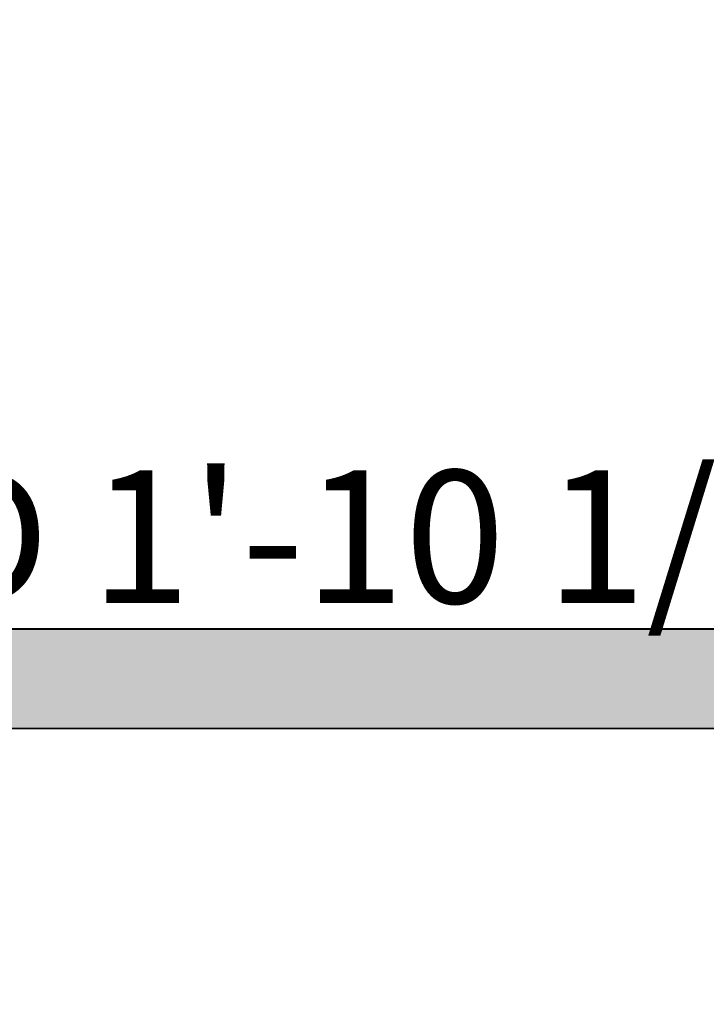
# Model space of a CAD drawing. Units: inches. Extents: x 2083 to 3317, y 1141 to 2115.
# Tile 118 of 256: x 2944 to 3006, y 1238 to 1327. Entities that reach past the tile are written whole.
import ezdxf

# ---------------------------------------------------------------- set-up
doc = ezdxf.new("R2010")
doc.units = ezdxf.units.IN
doc.layers.add('A-ANNO-DIMS', color=2, linetype='Continuous', lineweight=18)
doc.layers.add('A-WALL', color=7, linetype='Continuous', lineweight=35)
doc.layers.add('A-WALL-PATT', color=251, linetype='Continuous', lineweight=13, true_color=0x636466)
doc.styles.get("Standard").update_dxf_attribs({"font": 'arial.ttf'})
doc.dimstyles.new('ISO-25', dxfattribs={"dimtxt": 12, "dimasz": 12, "dimexe": 1.25, "dimexo": 0.625, "dimtad": 1, "dimlunit": 3, "dimtxsty": 'Standard', "dimcen": 2.5, "dimadec": 0, "dimazin": 0, "dimtfac": 1, "dimtmove": 0, "dimatfit": 3, "dimfxl": 1, "dimarcsym": 0})

# ---------------------------------------------------------------- blocks, each defined once
blk = doc.blocks.new('*D10')
at = {"layer": 'A-ANNO-DIMS', "color": 0, "lineweight": -2, "transparency": 16777216}
for p, q in [((2862.96, 1262.636), (2862.96, 1201.384)), ((3126.96, 1262.636), (3126.96, 1201.384)), ((2874.96, 1202.634), (3114.96, 1202.634))]:
    blk.add_line(p, q, dxfattribs=at)
at = {"layer": 'A-ANNO-DIMS', "color": 0, "transparency": 16777216}
for points in [[(2874.96, 1204.634), (2874.96, 1200.634), (2862.96, 1202.634)], [(3114.96, 1204.634), (3114.96, 1200.634), (3126.96, 1202.634)]]:
    blk.add_solid(points, dxfattribs=at)
at = {"layer": 'Defpoints', "color": 0, "transparency": 16777216}
for p in [(2862.96, 1263.261), (3126.96, 1263.261), (3126.96, 1202.634)]:
    blk.add_point(p, dxfattribs=at)
at = {"layer": 'A-ANNO-DIMS', "color": 0, "transparency": 16777216, "insert": (2994.96, 1209.284), "char_height": 12, "attachment_point": 5}
blk.add_mtext("22'", dxfattribs=at)
blk = doc.blocks.new('*D26')
at = {"layer": 'A-ANNO-DIMS', "color": 0, "lineweight": -2, "transparency": 16777216}
for p, q in [((3088.986, 1274.915), (3088.986, 1270.952)), ((3111.24, 1274.915), (3111.24, 1270.952)), ((3076.986, 1272.202), (2840.262, 1272.202)), ((3111.24, 1272.202), (3088.986, 1272.202)), ((3123.24, 1272.202), (3135.24, 1272.202))]:
    blk.add_line(p, q, dxfattribs=at)
at = {"layer": 'A-ANNO-DIMS', "color": 0, "transparency": 16777216}
for points in [[(3076.986, 1274.202), (3076.986, 1270.202), (3088.986, 1272.202)], [(3123.24, 1274.202), (3123.24, 1270.202), (3111.24, 1272.202)]]:
    blk.add_solid(points, dxfattribs=at)
at = {"layer": 'Defpoints', "color": 0, "transparency": 16777216}
for p in [(3088.986, 1275.54), (3111.24, 1275.54), (3088.986, 1272.202)]:
    blk.add_point(p, dxfattribs=at)
at = {"layer": 'A-ANNO-DIMS', "color": 0, "transparency": 16777216, "insert": (2952.624, 1279.032), "char_height": 12, "attachment_point": 5}
blk.add_mtext('NIGHTSTAND 1\'-10 1/2" TYP.', dxfattribs=at)
blk = doc.blocks.new('*D34')
at = {"layer": 'A-ANNO-DIMS', "color": 0, "lineweight": -2, "transparency": 16777216}
for p, q in [((2226.96, 1262.636), (2226.96, 1209.661)), ((3126.96, 1262.636), (3126.96, 1209.661)), ((2238.96, 1210.911), (3114.96, 1210.911))]:
    blk.add_line(p, q, dxfattribs=at)
at = {"layer": 'A-ANNO-DIMS', "color": 0, "transparency": 16777216}
for points in [[(2238.96, 1212.911), (2238.96, 1208.911), (2226.96, 1210.911)], [(3114.96, 1212.911), (3114.96, 1208.911), (3126.96, 1210.911)]]:
    blk.add_solid(points, dxfattribs=at)
at = {"layer": 'Defpoints', "color": 0, "transparency": 16777216}
for p in [(2226.96, 1263.261), (3126.96, 1263.261), (3126.96, 1210.911)]:
    blk.add_point(p, dxfattribs=at)
at = {"layer": 'A-ANNO-DIMS', "color": 0, "transparency": 16777216, "insert": (2676.96, 1217.663), "char_height": 12, "attachment_point": 5}
blk.add_mtext('75\'-0"', dxfattribs=at)

msp = doc.modelspace()

# ---------------------------------------------------------------- hatches: boundary and pattern name
at = {"layer": 'A-WALL-PATT'}
h = msp.add_hatch(color=256, dxfattribs=at)
h.dxf.hatch_style = 1
h.paths.add_polyline_path([(3126.96, 2020.761), (2748.96, 2020.761), (2604.96, 2020.761), (2226.96, 2020.761), (2226.96, 1702.761), (2466.96, 1702.761), (2466.96, 1582.761), (2418.96, 1582.761), (2418.96, 1477.761), (2226.96, 1477.761), (2226.96, 1263.261), (2544.96, 1263.261), (2544.96, 1411.761), (2604.96, 1411.761), (2685.96, 1411.761), (2685.96, 1420.761), (2604.96, 1420.761), (2604.96, 1573.761), (2604.96, 1702.761), (2604.96, 2011.761), (2748.96, 2011.761), (2748.96, 1702.761), (2862.96, 1702.761), (2862.96, 1621.761), (2871.96, 1621.761), (2871.96, 1702.761), (2883.96, 1702.761), (2883.96, 1706.939, -0.026459), (2883.96, 1711.761), (2757.96, 1711.761), (2757.96, 1807.761), (2787.96, 1807.761), (2787.96, 1812.261), (2757.96, 1812.261), (2757.96, 2011.761), (2877.96, 2011.761), (2877.96, 1812.261), (2847.96, 1812.261), (2847.96, 1807.761), (2889.836, 1807.761), (2889.836, 1812.261), (2882.46, 1812.261), (2882.46, 2011.761), (3117.96, 2011.761), (3117.96, 1812.261), (2937.836, 1812.261), (2937.836, 1807.761), (2995.71, 1807.761), (2995.71, 1796.118), (3000.21, 1796.118), (3000.21, 1807.761), (3117.96, 1807.761), (3117.96, 1711.761), (3000.21, 1711.761), (3000.21, 1760.118), (2998.573, 1760.118, -0.020711), (2995.71, 1760.118), (2995.71, 1711.761), (2931.96, 1711.761), (2931.96, 1702.761), (3126.96, 1702.761)])
h.paths.add_polyline_path([(2471.46, 2011.761), (2471.46, 1810.011), (2462.717, 1810.011), (2462.717, 1805.511), (2505.96, 1805.511), (2505.96, 1810.011), (2475.96, 1810.011), (2475.96, 2011.761), (2595.96, 2011.761), (2595.96, 1810.011), (2565.96, 1810.011), (2565.96, 1805.511), (2595.96, 1805.511), (2595.96, 1711.761), (2235.96, 1711.761), (2235.96, 1805.511), (2353.71, 1805.511), (2353.71, 1796.054), (2358.21, 1796.054), (2358.21, 1805.511), (2414.717, 1805.511), (2414.717, 1810.011), (2235.96, 1810.011), (2235.96, 2011.761)], flags=16)
h.paths.add_polyline_path([(2270.205, 1994.61), (2270.205, 1970.61), (2246.205, 1970.61), (2246.205, 1994.61)], flags=0)
edge = h.paths.add_edge_path(flags=0)
edge.add_ellipse((2332.027, 1899.798), major_axis=(-3.043, 3.043), ratio=0.168252, start_angle=-161.33217, end_angle=-156.30711, ccw=False)
edge.add_ellipse((2333.082, 1898.744), major_axis=(-1.055, 1.055), ratio=0.453532, start_angle=-123.37102, end_angle=-94.15911)
edge = h.paths.add_edge_path(flags=0)
edge.add_ellipse((2332.027, 1968.876), major_axis=(3.043, 3.043), ratio=0.168252, start_angle=18.66783, end_angle=23.69289)
edge.add_spline(control_points=[(2332.926, 1970.691), (2332.227, 1970.336), (2330.894, 1969.659), (2328.413, 1970.932), (2327.204, 1967.749), (2324.71, 1969.956), (2322.533, 1967.012), (2320.013, 1971.296), (2317.68, 1968.158), (2316.041, 1967.102), (2315.427, 1966.81)], knot_values=[0, 0, 0, 0, 2.267059, 4.324559, 6.685584, 8.878641, 11.121502, 14.300359, 17.755284, 19.732645, 19.732645, 19.732645, 19.732645], degree=3, periodic=0)
edge.add_ellipse((2332.027, 1968.876), major_axis=(3.043, 3.043), ratio=0.168252, start_angle=18.66783, end_angle=23.69289, ccw=False)
edge.add_ellipse((2333.082, 1969.931), major_axis=(1.055, 1.055), ratio=0.453532, start_angle=56.62898, end_angle=85.84089, ccw=False)
edge = h.paths.add_edge_path(flags=0)
edge.add_spline(control_points=[(2296.428, 1967.988), (2293.628, 1965.336), (2287.704, 1959.727), (2299.744, 1949.996), (2294.533, 1935.669), (2290.573, 1920.604), (2293.394, 1909.974), (2296.185, 1904.967)], knot_values=[0.099185, 0.099185, 0.099185, 0.099185, 0.345301, 0.619822, 0.982653, 1.386093, 1.810555, 1.810555, 1.810555, 1.810555], degree=3, periodic=0)
edge.add_spline(control_points=[(2296.185, 1904.967), (2297.384, 1902.619), (2298.001, 1901.949), (2298.553, 1901.468)], knot_values=[0.006246, 0.006246, 0.006246, 0.006246, 0.055476, 0.055476, 0.055476, 0.055476], degree=3, periodic=0)
edge.add_spline(control_points=[(2298.553, 1901.468), (2297.259, 1900.923), (2295.225, 1900.232), (2293.06, 1900.614), (2292.101, 1900.788), (2292.09, 1900.791)], knot_values=[0.312835, 0.312835, 0.312835, 0.312835, 0.40178, 0.474987, 0.475903, 0.475903, 0.475903, 0.475903], degree=3, periodic=0)
edge.add_arc((2292.794, 1904.664), 3.937, 215.4209, 259.69818, ccw=False)
edge.add_spline(control_points=[(2289.585, 1902.382), (2289.477, 1902.535), (2289.368, 1902.688), (2289.261, 1902.841)], knot_values=[0.102872, 0.102872, 0.102872, 0.102872, 0.116896, 0.116896, 0.116896, 0.116896], degree=3, periodic=0)
edge.add_spline(control_points=[(2289.261, 1902.841), (2288.687, 1902.55), (2287.64, 1902.02), (2285.881, 1901.874), (2283.853, 1901.504), (2281.72, 1899.711), (2278.467, 1899.493), (2276.157, 1901.883), (2272.259, 1899.804), (2267.778, 1901.843), (2262.244, 1900.184), (2257.415, 1901.782), (2254.318, 1900.726), (2253.178, 1900.337)], knot_values=[0, 0, 0, 0, 1.907977, 3.477176, 5.261074, 7.972851, 11.680248, 13.717921, 16.939592, 22.789562, 27.502503, 33.595215, 37.145618, 37.145618, 37.145618, 37.145618], degree=3, periodic=0)
edge.add_line((2253.178, 1900.337), (2250.244, 1902.841))
edge.add_line((2250.244, 1902.841), (2250.244, 1965.833))
edge.add_line((2250.244, 1965.833), (2253.178, 1968.337))
edge.add_spline(control_points=[(2253.178, 1968.337), (2254.318, 1967.948), (2257.415, 1966.892), (2262.244, 1968.49), (2267.778, 1966.831), (2271.527, 1968.537), (2273.876, 1967.828), (2274.207, 1967.728)], knot_values=[0, 0, 0, 0, 0.09018, 0.244935, 0.364644, 0.513233, 0.537855, 0.537855, 0.537855, 0.537855], degree=3, periodic=0)
edge.add_arc((2274.353, 1963.793), 3.937, 72.05113, 92.12795, ccw=False)
edge.add_arc((2281.297, 1985.23), 18.596, 252.05113, 288.56572)
edge.add_arc((2292.317, 1956.029), 12.646, 71.02679, 113.77822, ccw=False)
edge = h.paths.add_edge_path(flags=0)
edge.add_spline(control_points=[(2274.899, 1951.856), (2275.066, 1951.617), (2275.233, 1951.377), (2275.398, 1951.136)], knot_values=[1.409916, 1.409916, 1.409916, 1.409916, 1.43159, 1.43159, 1.43159, 1.43159], degree=3, periodic=0)
edge.add_spline(control_points=[(2275.398, 1951.136), (2275.792, 1950.562), (2276.179, 1949.984), (2276.546, 1949.397)], knot_values=[1.358238, 1.358238, 1.358238, 1.358238, 1.409916, 1.409916, 1.409916, 1.409916], degree=3, periodic=0)
edge.add_line((2276.546, 1949.397), (2277.437, 1947.862))
edge.add_spline(control_points=[(2277.437, 1947.862), (2276.304, 1945.673), (2274.64, 1942.427), (2274.632, 1938.094), (2272.799, 1930.852), (2274.356, 1943.897), (2275.948, 1947.923), (2276.546, 1949.397)], knot_values=[0.005632, 0.005632, 0.005632, 0.005632, 0.186014, 0.266002, 0.357087, 0.59639, 0.739732, 0.739732, 0.739732, 0.739732], degree=3, periodic=0)
edge.add_spline(control_points=[(2276.546, 1949.397), (2276.179, 1949.984), (2275.792, 1950.562), (2275.398, 1951.136)], knot_values=[1.358238, 1.358238, 1.358238, 1.358238, 1.409916, 1.409916, 1.409916, 1.409916], degree=3, periodic=0)
edge.add_spline(control_points=[(2275.398, 1951.136), (2274.943, 1950.08), (2274.208, 1948.025), (2273.935, 1944.851), (2272.469, 1937.627), (2273.466, 1945.696), (2274.701, 1951.059), (2274.899, 1951.856)], knot_values=[0.104364, 0.104364, 0.104364, 0.104364, 0.189636, 0.269624, 0.36071, 0.600013, 0.644622, 0.644622, 0.644622, 0.644622], degree=3, periodic=0)
h.paths.add_polyline_path([(2269.168, 1963.128, -0.357527), (2268.171, 1960.976, -0.092561), (2268.171, 1939.436, -0.357527), (2269.168, 1937.285, -0.357527), (2267.016, 1938.282, -0.164785), (2254.686, 1938.282, -0.357527), (2252.534, 1937.285, -0.357527), (2253.531, 1939.436, -0.092561), (2253.531, 1960.976, -0.357527), (2252.534, 1963.128, -0.357527), (2254.686, 1962.131, -0.164785), (2267.016, 1962.131, -0.357527)], flags=0)
h.paths.add_polyline_path([(2248.874, 1967.802), (2248.874, 1957.028), (2249.458, 1957.028), (2249.458, 1911.647), (2248.874, 1911.647), (2248.874, 1900.873), (2246.512, 1900.873, 0.197327), (2244.15, 1902.457), (2244.15, 1966.218, 0.197327), (2246.512, 1967.802)], flags=0)
h.paths.add_polyline_path([(2269.168, 1931.389, -0.357527), (2268.171, 1929.238, -0.092561), (2268.171, 1907.698, -0.357527), (2269.168, 1905.547, -0.357527), (2267.016, 1906.544, -0.164785), (2254.686, 1906.544, -0.357527), (2252.534, 1905.547, -0.357527), (2253.531, 1907.698, -0.092561), (2253.531, 1929.238, -0.357527), (2252.534, 1931.389, -0.357527), (2254.686, 1930.392, -0.164785), (2267.016, 1930.392, -0.357527)], flags=0)
edge = h.paths.add_edge_path(flags=0)
edge.add_spline(control_points=[(2276.197, 1906.724), (2276.168, 1909.029), (2276.114, 1913.372), (2270.598, 1924.925), (2273.905, 1919.013), (2275.922, 1916.262), (2275.475, 1912.402), (2277.258, 1910.381), (2276.696, 1908.225), (2276.646, 1906.813), (2276.618, 1906.008)], knot_values=[0, 0, 0, 0, 8.61026, 16.221274, 18.843057, 23.804898, 27.440828, 29.356102, 31.203478, 33.650687, 33.650687, 33.650687, 33.650687], degree=3, periodic=0)
edge.add_spline(control_points=[(2276.618, 1906.008), (2276.623, 1905.624), (2276.498, 1904.629), (2275.442, 1903.855), (2274.937, 1903.08), (2274.859, 1902.841)], knot_values=[0.156488, 0.156488, 0.156488, 0.156488, 0.184398, 0.231376, 0.250598, 0.250598, 0.250598, 0.250598], degree=3, periodic=0)
edge.add_line((2274.859, 1902.841), (2276.506, 1902.841))
edge.add_spline(control_points=[(2276.506, 1902.841), (2276.788, 1903.085), (2277.665, 1904.125), (2278.25, 1904.341), (2277.654, 1908.527), (2278.156, 1906.228), (2278.1, 1905.286), (2278.847, 1904.069), (2277.857, 1903.415), (2277.874, 1902.991), (2277.904, 1902.841)], knot_values=[0.059574, 0.059574, 0.059574, 0.059574, 0.080753, 0.103741, 0.16972, 0.176036, 0.207137, 0.240474, 0.262341, 0.27366, 0.27366, 0.27366, 0.27366], degree=3, periodic=0)
edge.add_line((2277.904, 1902.841), (2280.03, 1902.841))
edge.add_spline(control_points=[(2280.03, 1902.841), (2279.888, 1903.088), (2279.499, 1903.982), (2280.152, 1905.939), (2278.104, 1909.658), (2279.762, 1907.185), (2280.328, 1904.875), (2280.485, 1903.49), (2281.463, 1903.249), (2281.758, 1902.936), (2281.834, 1902.841)], knot_values=[0.013856, 0.013856, 0.013856, 0.013856, 0.034874, 0.088867, 0.107879, 0.126738, 0.158714, 0.193757, 0.217487, 0.226722, 0.226722, 0.226722, 0.226722], degree=3, periodic=0)
edge.add_spline(control_points=[(2281.834, 1902.841), (2281.788, 1902.827), (2281.647, 1902.783), (2281.396, 1902.859), (2281.088, 1902.985), (2280.721, 1903.061), (2280.333, 1903.026), (2280.125, 1902.899), (2280.03, 1902.841)], knot_values=[0, 0, 0, 0, 0.14413, 0.435517, 0.749276, 1.153046, 1.548371, 1.878348, 1.878348, 1.878348, 1.878348], degree=3, periodic=0)
edge.add_line((2280.03, 1902.841), (2277.904, 1902.841))
edge.add_spline(control_points=[(2277.904, 1902.841), (2277.893, 1902.796), (2277.865, 1902.68), (2277.607, 1902.687), (2277.274, 1902.801), (2276.838, 1902.62), (2276.584, 1902.789), (2276.506, 1902.841)], knot_values=[0, 0, 0, 0, 0.127189, 0.326199, 0.628009, 1.24357, 1.515331, 1.515331, 1.515331, 1.515331], degree=3, periodic=0)
edge.add_line((2276.506, 1902.841), (2274.859, 1902.841))
edge.add_spline(control_points=[(2274.859, 1902.841), (2274.814, 1902.899), (2274.725, 1903.013), (2274.493, 1903.119), (2274.244, 1902.961), (2273.937, 1903.185), (2273.614, 1902.983), (2273.408, 1902.883), (2273.322, 1902.841)], knot_values=[0, 0, 0, 0, 0.21843, 0.436957, 0.687977, 0.990379, 1.398396, 1.69185, 1.69185, 1.69185, 1.69185], degree=3, periodic=0)
edge.add_spline(control_points=[(2273.322, 1902.841), (2273.617, 1903.446), (2274.274, 1904.538), (2276.027, 1904.574), (2276.207, 1906.584), (2276.197, 1906.724)], knot_values=[0.012227, 0.012227, 0.012227, 0.012227, 0.059472, 0.106218, 0.134458, 0.134458, 0.134458, 0.134458], degree=3, periodic=0)
h.paths.add_polyline_path([(2270.776, 1897.79), (2270.776, 1873.79), (2246.776, 1873.79), (2246.776, 1897.79)], flags=0)
h.paths.add_polyline_path([(2353.71, 1760.005), (2353.71, 1760.054), (2358.21, 1760.054, -0.033729)], flags=0)
h.paths.add_polyline_path([(2321.819, 1737.529), (2341.995, 1737.529, -0.414214), (2343.203, 1736.321), (2343.203, 1721.021, -0.414214), (2341.995, 1719.813), (2321.819, 1719.813, -0.414214), (2320.611, 1721.021), (2320.611, 1736.321, -0.414214)], flags=0)
h.paths.add_polyline_path([(2324.235, 1736.321), (2339.579, 1736.321, -0.414214), (2341.995, 1733.905), (2341.995, 1725.45, -0.414214), (2339.579, 1723.034), (2333.681, 1723.034), (2333.845, 1722.045, -0.870646), (2335.425, 1721.826, -0.767327), (2333.923, 1721.423), (2331.291, 1721.423, -0.767327), (2329.788, 1721.826, -0.870646), (2331.368, 1722.045), (2331.533, 1723.034), (2324.235, 1723.034, -0.414214), (2321.819, 1725.45), (2321.819, 1733.905, -0.414214)], flags=0)
h.paths.add_polyline_path([(2570.484, 1928.615), (2589.684, 1928.615), (2590.169, 1928.615), (2590.169, 1904.993), (2570.484, 1904.993)], flags=0)
h.paths.add_polyline_path([(2574.447, 1927.264, -1), (2572.829, 1927.264, -1)], flags=0)
h.paths.add_polyline_path([(2573.09, 1926.941), (2573.925, 1927.776), (2574.148, 1927.553), (2573.313, 1926.718)], flags=0)
h.paths.add_polyline_path([(2578.779, 1919.73, -1), (2571.592, 1919.73, -1)], flags=0)
h.paths.add_polyline_path([(2578.385, 1919.73, -1), (2571.985, 1919.73, -1)], flags=0)
h.paths.add_polyline_path([(2331.596, 1729.476, -1), (2333.618, 1729.476, -1)], flags=0)
h.paths.add_polyline_path([(2578.034, 1927.264, -1), (2576.416, 1927.264, -1)], flags=0)
h.paths.add_polyline_path([(2576.689, 1927.531), (2576.912, 1927.754), (2577.747, 1926.919), (2577.524, 1926.696)], flags=0)
h.paths.add_polyline_path([(2578.139, 1909.86, -1), (2572.232, 1909.86, -1)], flags=0)
h.paths.add_polyline_path([(2577.745, 1909.86, -1), (2572.625, 1909.86, -1)], flags=0)
h.paths.add_polyline_path([(2583.798, 1927.264, -1), (2582.179, 1927.264, -1)], flags=0)
h.paths.add_polyline_path([(2582.719, 1927.754), (2583.554, 1926.919), (2583.331, 1926.696), (2582.496, 1927.531)], flags=0)
h.paths.add_polyline_path([(2582.496, 1927.531), (2582.719, 1927.754), (2583.554, 1926.919), (2583.331, 1926.696)], flags=0)
h.paths.add_polyline_path([(2587.739, 1920.53, -1), (2581.832, 1920.53, -1)], flags=0)
h.paths.add_polyline_path([(2587.345, 1920.53, -1), (2582.225, 1920.53, -1)], flags=0)
h.paths.add_polyline_path([(2587.385, 1927.264, -1), (2585.766, 1927.264, -1)], flags=0)
h.paths.add_polyline_path([(2586.082, 1926.98), (2586.917, 1927.815), (2587.14, 1927.593), (2586.305, 1926.758)], flags=0)
h.paths.add_polyline_path([(2588.379, 1910.66, -1), (2581.192, 1910.66, -1)], flags=0)
h.paths.add_polyline_path([(2587.985, 1910.66, -1), (2581.585, 1910.66, -1)], flags=0)
h.paths.add_polyline_path([(2417.168, 1729.478), (2437.344, 1729.478, -0.414214), (2438.552, 1728.27), (2438.552, 1712.969, -0.414214), (2437.344, 1711.761), (2417.168, 1711.761, -0.414214), (2415.96, 1712.969), (2415.96, 1728.27, -0.414214)], flags=0)
h.paths.add_polyline_path([(2419.584, 1728.27), (2434.928, 1728.27, -0.414214), (2437.344, 1725.854), (2437.344, 1717.398, -0.414214), (2434.928, 1714.983), (2429.029, 1714.983), (2429.194, 1713.994, -0.870646), (2430.774, 1713.775, -0.767327), (2429.271, 1713.372), (2426.64, 1713.372, -0.767327), (2425.137, 1713.775, -0.870646), (2426.717, 1713.994), (2426.882, 1714.983), (2419.584, 1714.983, -0.414214), (2417.168, 1717.398), (2417.168, 1725.854, -0.414214)], flags=0)
h.paths.add_polyline_path([(2419.584, 1728.27), (2434.928, 1728.27, -0.414214), (2437.344, 1725.854), (2437.344, 1717.398, -0.414214), (2434.928, 1714.983), (2429.029, 1714.983), (2428.358, 1719.009), (2427.553, 1719.009), (2426.882, 1714.983), (2419.584, 1714.983, -0.414214), (2417.168, 1717.398), (2417.168, 1725.854, -0.414214)], flags=0)
h.paths.add_polyline_path([(2426.944, 1721.425, -1), (2428.967, 1721.425, -1)], flags=0)
h.paths.add_polyline_path([(2475.96, 1702.761), (2595.96, 1702.761), (2595.96, 1582.761), (2475.96, 1582.761)], flags=16)
h.paths.add_polyline_path([(2427.96, 1573.761), (2595.96, 1573.761), (2595.96, 1468.761), (2595.96, 1420.761), (2384.46, 1420.761), (2384.46, 1468.761), (2427.96, 1468.761)], flags=16)
h.paths.add_polyline_path([(2379.96, 1468.761), (2379.96, 1420.761), (2235.96, 1420.761), (2235.96, 1468.761)], flags=16)
h.paths.add_polyline_path([(2317.816, 1466.696), (2337.992, 1466.696, -0.414214), (2339.2, 1465.488), (2339.2, 1450.187, -0.414214), (2337.992, 1448.979), (2317.816, 1448.979, -0.414214), (2316.608, 1450.187), (2316.608, 1465.488, -0.414214)], flags=0)
h.paths.add_polyline_path([(2320.232, 1465.488), (2335.576, 1465.488, -0.414214), (2337.992, 1463.072), (2337.992, 1454.616, -0.414214), (2335.576, 1452.2), (2329.677, 1452.2), (2329.842, 1451.212, -0.870646), (2331.422, 1450.992, -0.767327), (2329.92, 1450.59), (2327.288, 1450.59, -0.767327), (2325.785, 1450.992, -0.870646), (2327.365, 1451.212), (2327.53, 1452.2), (2320.232, 1452.2, -0.414214), (2317.816, 1454.616), (2317.816, 1463.072, -0.414214)], flags=0)
h.paths.add_polyline_path([(2320.232, 1465.488), (2335.576, 1465.488, -0.414214), (2337.992, 1463.072), (2337.992, 1454.616, -0.414214), (2335.576, 1452.2), (2329.677, 1452.2), (2329.006, 1456.227), (2328.201, 1456.227), (2327.53, 1452.2), (2320.232, 1452.2, -0.414214), (2317.816, 1454.616), (2317.816, 1463.072, -0.414214)], flags=0)
h.paths.add_polyline_path([(2327.593, 1458.643, -1), (2329.615, 1458.643, -1)], flags=0)
h.paths.add_polyline_path([(2244.412, 1433.34), (2241.921, 1433.34, -0.414214), (2240.018, 1435.244), (2240.018, 1440.953, -0.414211), (2241.921, 1442.856), (2244.412, 1442.856, -1.976472)], flags=0)
h.paths.add_polyline_path([(2245.357, 1434.398, -0.414214), (2245.357, 1441.799, -2.144098)], flags=0)
h.paths.add_polyline_path([(2535.96, 1416.261), (2535.96, 1272.261), (2235.96, 1272.261), (2235.96, 1416.261)], flags=16)
h.paths.add_polyline_path([(2260.12, 1384.293), (2260.12, 1362.039), (2237.865, 1362.039), (2237.865, 1384.293)], flags=0)
edge = h.paths.add_edge_path(flags=0)
edge.add_line((2318.252, 1362.093), (2318.146, 1362.001))
edge.add_ellipse((2317.445, 1360.431), major_axis=(2.822, 2.822), ratio=0.168252, start_angle=18.66783, end_angle=20.94813, ccw=False)
edge.add_ellipse((2318.423, 1361.409), major_axis=(0.978, 0.978), ratio=0.453532, start_angle=56.62898, end_angle=70.2262, ccw=False)
edge = h.paths.add_edge_path(flags=0)
edge.add_line((2319.107, 1295.571), (2319.015, 1295.677))
edge.add_ellipse((2317.445, 1296.378), major_axis=(-2.822, 2.822), ratio=0.168252, start_angle=-161.33217, end_angle=-159.05187, ccw=False)
edge.add_ellipse((2318.423, 1295.4), major_axis=(-0.978, 0.978), ratio=0.453532, start_angle=-123.37102, end_angle=-109.7738)
edge = h.paths.add_edge_path(flags=0)
edge.add_spline(control_points=[(2284.21, 1301.17), (2284.581, 1300.445), (2284.891, 1299.892), (2285.16, 1299.461)], knot_values=[0.039066, 0.039066, 0.039066, 0.039066, 0.055476, 0.055476, 0.055476, 0.055476], degree=3, periodic=0)
edge.add_line((2285.16, 1299.461), (2284.21, 1301.17))
edge = h.paths.add_edge_path(flags=0)
edge.add_line((2280.412, 1297.298), (2283.37, 1297.036))
edge.add_line((2283.37, 1297.036), (2286.406, 1297.926))
edge.add_spline(control_points=[(2286.406, 1297.926), (2285.305, 1297.463), (2284.345, 1297.129), (2283.37, 1297.036)], knot_values=[0.394369, 0.394369, 0.394369, 0.394369, 0.475903, 0.475903, 0.475903, 0.475903], degree=3, periodic=0)
edge.add_spline(control_points=[(2283.37, 1297.036), (2283.281, 1297.028), (2282.316, 1296.957), (2281.313, 1297.134), (2280.423, 1297.296), (2280.412, 1297.298)], knot_values=[0.312835, 0.312835, 0.312835, 0.312835, 0.320246, 0.393453, 0.394369, 0.394369, 0.394369, 0.394369], degree=3, periodic=0)
edge = h.paths.add_edge_path(flags=0)
edge.add_line((2284.436, 1359.607), (2280.446, 1355.328))
edge.add_line((2280.446, 1355.328), (2279.58, 1351.018))
edge.add_line((2279.58, 1351.018), (2282.413, 1346.58))
edge.add_spline(control_points=[(2282.413, 1346.58), (2283.153, 1345.589), (2284.253, 1344.029), (2284.801, 1342.387), (2284.935, 1341.806)], knot_values=[1.240098, 1.240098, 1.240098, 1.240098, 1.332892, 1.382712, 1.382712, 1.382712, 1.382712], degree=3, periodic=0)
edge.add_spline(control_points=[(2284.935, 1341.806), (2285.319, 1340.141), (2285.233, 1338.409), (2284.91, 1336.654)], knot_values=[1.097484, 1.097484, 1.097484, 1.097484, 1.240098, 1.240098, 1.240098, 1.240098], degree=3, periodic=0)
edge.add_spline(control_points=[(2284.91, 1336.654), (2284.587, 1334.899), (2284.027, 1333.12), (2283.463, 1331.361)], knot_values=[0.95487, 0.95487, 0.95487, 0.95487, 1.097484, 1.097484, 1.097484, 1.097484], degree=3, periodic=0)
edge.add_line((2283.463, 1331.361), (2281.89, 1326.153))
edge.add_line((2281.89, 1326.153), (2280.756, 1321.056))
edge.add_line((2280.756, 1321.056), (2280.299, 1316.002))
edge.add_line((2280.299, 1316.002), (2280.716, 1310.95))
edge.add_line((2280.716, 1310.95), (2282.028, 1305.972))
edge.add_line((2282.028, 1305.972), (2284.21, 1301.17))
edge.add_spline(control_points=[(2284.21, 1301.17), (2283.341, 1302.73), (2282.612, 1304.336), (2282.028, 1305.972)], knot_values=[0.099185, 0.099185, 0.099185, 0.099185, 0.241799, 0.241799, 0.241799, 0.241799], degree=3, periodic=0)
edge.add_spline(control_points=[(2282.028, 1305.972), (2281.444, 1307.608), (2281.005, 1309.273), (2280.716, 1310.95)], knot_values=[0.241799, 0.241799, 0.241799, 0.241799, 0.384413, 0.384413, 0.384413, 0.384413], degree=3, periodic=0)
edge.add_spline(control_points=[(2280.716, 1310.95), (2280.433, 1312.588), (2280.289, 1314.277), (2280.299, 1315.962), (2280.299, 1316.002)], knot_values=[0.384413, 0.384413, 0.384413, 0.384413, 0.523647, 0.527028, 0.527028, 0.527028, 0.527028], degree=3, periodic=0)
edge.add_spline(control_points=[(2280.299, 1316.002), (2280.312, 1317.687), (2280.478, 1319.368), (2280.756, 1321.056)], knot_values=[0.527028, 0.527028, 0.527028, 0.527028, 0.669642, 0.669642, 0.669642, 0.669642], degree=3, periodic=0)
edge.add_spline(control_points=[(2280.756, 1321.056), (2281.035, 1322.744), (2281.426, 1324.44), (2281.89, 1326.153)], knot_values=[0.669642, 0.669642, 0.669642, 0.669642, 0.812256, 0.812256, 0.812256, 0.812256], degree=3, periodic=0)
edge.add_spline(control_points=[(2281.89, 1326.153), (2282.264, 1327.533), (2282.788, 1329.262), (2283.353, 1331.018), (2283.463, 1331.361)], knot_values=[0.812256, 0.812256, 0.812256, 0.812256, 0.927087, 0.95487, 0.95487, 0.95487, 0.95487], degree=3, periodic=0)
edge.add_line((2283.463, 1331.361), (2284.91, 1336.654))
edge.add_line((2284.91, 1336.654), (2284.935, 1341.806))
edge.add_line((2284.935, 1341.806), (2282.413, 1346.58))
edge.add_spline(control_points=[(2282.413, 1346.58), (2281.275, 1348.104), (2280.078, 1349.57), (2279.58, 1351.018)], knot_values=[1.382712, 1.382712, 1.382712, 1.382712, 1.525326, 1.525326, 1.525326, 1.525326], degree=3, periodic=0)
edge.add_spline(control_points=[(2279.58, 1351.018), (2279.443, 1351.415), (2279.136, 1352.857), (2279.735, 1354.29), (2280.446, 1355.328)], knot_values=[1.525326, 1.525326, 1.525326, 1.525326, 1.564439, 1.667941, 1.667941, 1.667941, 1.667941], degree=3, periodic=0)
edge.add_spline(control_points=[(2280.446, 1355.328), (2281.426, 1356.758), (2282.931, 1358.183), (2284.436, 1359.607)], knot_values=[1.667941, 1.667941, 1.667941, 1.667941, 1.810555, 1.810555, 1.810555, 1.810555], degree=3, periodic=0)
edge.add_arc((2280.623, 1348.518), 11.726, 71.02679, 113.77822)
edge.add_arc((2270.405, 1375.595), 17.244, 252.05113, 288.56572, ccw=False)
edge.add_arc((2263.966, 1355.718), 3.651, 72.05113, 92.12795)
edge.add_arc((2263.966, 1355.718), 3.651, 92.12795, 177.98513)
edge.add_spline(control_points=[(2260.318, 1355.846), (2260.26, 1354.221), (2260.551, 1350.187), (2262.999, 1346.766), (2264.473, 1344.649)], knot_values=[1.43159, 1.43159, 1.43159, 1.43159, 1.564144, 1.770695, 1.770695, 1.770695, 1.770695], degree=3, periodic=0)
edge.add_line((2264.473, 1344.649), (2264.936, 1343.983))
edge.add_spline(control_points=[(2263.801, 1340.248), (2263.843, 1340.514), (2264.067, 1341.756), (2264.513, 1343.002), (2264.935, 1343.981)], knot_values=[0.53657, 0.53657, 0.53657, 0.53657, 0.559349, 0.644622, 0.644622, 0.644622, 0.644622], degree=3, periodic=0)
edge.add_spline(control_points=[(2264.935, 1343.981), (2265.118, 1343.715), (2265.299, 1343.448), (2265.477, 1343.179)], knot_values=[1.384077, 1.384077, 1.384077, 1.384077, 1.409916, 1.409916, 1.409916, 1.409916], degree=3, periodic=0)
edge.add_spline(control_points=[(2265.477, 1343.179), (2265.655, 1342.911), (2265.829, 1342.641), (2265.999, 1342.369)], knot_values=[1.358238, 1.358238, 1.358238, 1.358238, 1.384077, 1.384077, 1.384077, 1.384077], degree=3, periodic=0)
edge.add_line((2265.999, 1342.369), (2266.826, 1340.946))
edge.add_spline(control_points=[(2266.826, 1340.946), (2268.894, 1337.09), (2271.398, 1325.843), (2270.516, 1310.569), (2275.919, 1301.861), (2277.79, 1299.199)], knot_values=[0.116896, 0.116896, 0.116896, 0.116896, 0.472987, 1.050969, 1.313793, 1.313793, 1.313793, 1.313793], degree=3, periodic=0)
edge.add_spline(control_points=[(2277.79, 1299.199), (2277.839, 1299.128), (2277.889, 1299.057), (2277.94, 1298.987)], knot_values=[0.109884, 0.109884, 0.109884, 0.109884, 0.116896, 0.116896, 0.116896, 0.116896], degree=3, periodic=0)
edge.add_line((2277.94, 1298.987), (2277.789, 1299.199))
edge.add_spline(control_points=[(2277.789, 1299.199), (2277.257, 1298.929), (2276.286, 1298.438), (2275.039, 1298.334), (2274.383, 1298.239), (2274.215, 1298.209)], knot_values=[33.12187, 33.12187, 33.12187, 33.12187, 35.029056, 36.598255, 37.144827, 37.144827, 37.144827, 37.144827], degree=3, periodic=0)
edge.add_line((2274.215, 1298.209), (2273.073, 1297.893))
edge.add_spline(control_points=[(2273.073, 1297.893), (2272.323, 1297.58), (2271.039, 1296.511), (2269.248, 1296.226), (2268.423, 1296.375)], knot_values=[26.532584, 26.532584, 26.532584, 26.532584, 29.198919, 31.839101, 31.839101, 31.839101, 31.839101], degree=3, periodic=0)
edge.add_line((2268.423, 1296.375), (2263.879, 1297.458))
edge.add_spline(control_points=[(2263.879, 1297.458), (2263.556, 1297.359), (2261.86, 1296.839), (2260.239, 1297.282), (2258.933, 1297.516)], knot_values=[15.919551, 15.919551, 15.919551, 15.919551, 16.939592, 21.226067, 21.226067, 21.226067, 21.226067], degree=3, periodic=0)
edge.add_line((2258.933, 1297.516), (2254.055, 1297.329))
edge.add_spline(control_points=[(2254.055, 1297.329), (2253.756, 1297.296), (2252.114, 1297.165), (2250.462, 1297.544), (2249.13, 1297.668)], knot_values=[5.306517, 5.306517, 5.306517, 5.306517, 6.276435, 10.613034, 10.613034, 10.613034, 10.613034], degree=3, periodic=0)
edge.add_line((2249.13, 1297.668), (2244.332, 1296.878))
edge.add_line((2244.332, 1296.878), (2241.611, 1299.199))
edge.add_line((2241.611, 1299.199), (2241.611, 1357.609))
edge.add_line((2241.611, 1357.609), (2244.332, 1359.931))
edge.add_line((2244.332, 1359.931), (2252.729, 1359.543))
edge.add_spline(control_points=[(2252.729, 1359.543), (2252.871, 1359.546), (2253.306, 1359.548), (2253.74, 1359.514), (2254.032, 1359.482)], knot_values=[0.233291, 0.233291, 0.233291, 0.233291, 0.244935, 0.268927, 0.268927, 0.268927, 0.268927], degree=3, periodic=0)
edge.add_line((2254.032, 1359.482), (2259.587, 1359.416))
edge.add_spline(control_points=[(2259.587, 1359.416), (2260.677, 1359.629), (2262.073, 1359.897), (2263.524, 1359.459), (2263.83, 1359.366)], knot_values=[0.422516, 0.422516, 0.422516, 0.422516, 0.513233, 0.537855, 0.537855, 0.537855, 0.537855], degree=3, periodic=0)
edge.add_arc((2263.966, 1355.718), 3.651, 72.05113, 92.12795, ccw=False)
edge.add_arc((2270.405, 1375.595), 17.244, 252.05113, 288.56572)
edge.add_arc((2280.623, 1348.518), 11.726, 71.02679, 113.77822, ccw=False)
h.paths.add_polyline_path([(2240.341, 1359.435), (2240.341, 1349.444), (2240.882, 1349.444), (2240.882, 1307.365), (2240.341, 1307.365), (2240.341, 1297.374), (2238.15, 1297.374, 0.197327), (2235.96, 1298.843), (2235.96, 1357.966, 0.197327), (2238.15, 1359.435)], flags=0)
h.paths.add_polyline_path([(2259.158, 1355.101, -0.357527), (2258.233, 1353.106, -0.092561), (2258.233, 1333.133, -0.357527), (2259.158, 1331.138, -0.357527), (2257.163, 1332.062, -0.164785), (2245.729, 1332.062, -0.357527), (2243.735, 1331.138, -0.357527), (2244.659, 1333.133, -0.092561), (2244.659, 1353.106, -0.357527), (2243.735, 1355.101, -0.357527), (2245.729, 1354.176, -0.164785), (2257.163, 1354.176, -0.357527)], flags=0)
edge = h.paths.add_edge_path(flags=0)
edge.add_line((2265.999, 1342.369), (2266.826, 1340.946))
edge.add_line((2266.826, 1340.946), (2265.308, 1337.814))
edge.add_line((2265.308, 1337.814), (2264.358, 1334.653))
edge.add_line((2264.358, 1334.653), (2264.262, 1333.8))
edge.add_spline(control_points=[(2264.262, 1333.8), (2264.208, 1333.187), (2264.162, 1332.366), (2264.007, 1331.414), (2263.969, 1331.202)], knot_values=[0.464444, 0.464444, 0.464444, 0.464444, 0.516691, 0.531608, 0.531608, 0.531608, 0.531608], degree=3, periodic=0)
edge.add_spline(control_points=[(2263.969, 1331.202), (2263.775, 1330.119), (2263.424, 1328.791), (2263.257, 1328.531), (2263.234, 1328.515)], knot_values=[0.372682, 0.372682, 0.372682, 0.372682, 0.44885, 0.464444, 0.464444, 0.464444, 0.464444], degree=3, periodic=0)
edge.add_spline(control_points=[(2263.234, 1328.515), (2263.096, 1328.42), (2263.131, 1329.301), (2263.275, 1330.616)], knot_values=[0.280919, 0.280919, 0.280919, 0.280919, 0.372682, 0.372682, 0.372682, 0.372682], degree=3, periodic=0)
edge.add_spline(control_points=[(2263.275, 1330.616), (2263.419, 1331.93), (2263.672, 1333.677), (2263.97, 1335.315)], knot_values=[0.189157, 0.189157, 0.189157, 0.189157, 0.280919, 0.280919, 0.280919, 0.280919], degree=3, periodic=0)
edge.add_spline(control_points=[(2263.97, 1335.315), (2264.1, 1336.032), (2264.419, 1337.622), (2264.755, 1338.864), (2264.947, 1339.491)], knot_values=[0.097394, 0.097394, 0.097394, 0.097394, 0.137578, 0.189157, 0.189157, 0.189157, 0.189157], degree=3, periodic=0)
edge.add_spline(control_points=[(2264.947, 1339.491), (2265.29, 1340.606), (2265.644, 1341.494), (2265.999, 1342.369)], knot_values=[0.005632, 0.005632, 0.005632, 0.005632, 0.097394, 0.097394, 0.097394, 0.097394], degree=3, periodic=0)
h.paths.add_polyline_path([(2259.158, 1325.671, -0.357527), (2258.233, 1323.676, -0.092561), (2258.233, 1303.703, -0.357527), (2259.158, 1301.708, -0.357527), (2257.163, 1302.633, -0.164785), (2245.729, 1302.633, -0.357527), (2243.735, 1301.708, -0.357527), (2244.659, 1303.703, -0.092561), (2244.659, 1323.676, -0.357527), (2243.735, 1325.671, -0.357527), (2245.729, 1324.747, -0.164785), (2257.163, 1324.747, -0.357527)], flags=0)
edge = h.paths.add_edge_path(flags=0)
edge.add_spline(control_points=[(2261.709, 1317.311), (2261.679, 1317.418), (2261.762, 1317.389), (2262.491, 1316.09), (2262.962, 1315.301)], knot_values=[14.955861, 14.955861, 14.955861, 14.955861, 16.221274, 18.694826, 18.694826, 18.694826, 18.694826], degree=3, periodic=0)
edge.add_spline(control_points=[(2262.962, 1315.301), (2262.99, 1315.254), (2263.702, 1314.067), (2264.349, 1313.127), (2264.73, 1312.164)], knot_values=[18.694826, 18.694826, 18.694826, 18.694826, 18.843057, 22.433791, 22.433791, 22.433791, 22.433791], degree=3, periodic=0)
edge.add_spline(control_points=[(2264.73, 1312.164), (2264.876, 1311.796), (2265.177, 1310.77), (2265.143, 1309.559), (2265.248, 1308.824)], knot_values=[22.433791, 22.433791, 22.433791, 22.433791, 23.804898, 26.172756, 26.172756, 26.172756, 26.172756], degree=3, periodic=0)
edge.add_line((2265.248, 1308.824), (2265.851, 1307.172))
edge.add_spline(control_points=[(2265.851, 1307.172), (2266.065, 1306.822), (2266.384, 1306.332), (2266.424, 1305.781), (2266.42, 1305.611)], knot_values=[28.062562, 28.062562, 28.062562, 28.062562, 29.356102, 29.911721, 29.911721, 29.911721, 29.911721], degree=3, periodic=0)
edge.add_spline(control_points=[(2266.42, 1305.611), (2266.416, 1305.433), (2266.394, 1305.25), (2266.365, 1305.066)], knot_values=[29.911721, 29.911721, 29.911721, 29.911721, 30.497837, 30.497837, 30.497837, 30.497837], degree=3, periodic=0)
edge.add_line((2266.365, 1305.066), (2266.066, 1302.136))
edge.add_spline(control_points=[(2266.066, 1302.136), (2266.071, 1301.78), (2265.998, 1301.2), (2265.663, 1300.759), (2265.509, 1300.586)], knot_values=[0.156488, 0.156488, 0.156488, 0.156488, 0.184398, 0.203543, 0.203543, 0.203543, 0.203543], degree=3, periodic=0)
edge.add_line((2265.509, 1300.586), (2264.435, 1299.199))
edge.add_line((2264.435, 1299.199), (2265.962, 1299.199))
edge.add_line((2265.962, 1299.199), (2267.336, 1301.175))
edge.add_line((2267.336, 1301.175), (2267.312, 1301.986))
edge.add_spline(control_points=[(2267.312, 1301.986), (2267.261, 1302.862), (2267.16, 1303.737), (2267.271, 1303.326)], knot_values=[0.126229, 0.126229, 0.126229, 0.126229, 0.166617, 0.166617, 0.166617, 0.166617], degree=3, periodic=0)
edge.add_spline(control_points=[(2267.271, 1303.326), (2267.28, 1303.294), (2267.31, 1303.175), (2267.373, 1302.884), (2267.406, 1302.683), (2267.418, 1302.601)], knot_values=[0.166617, 0.166617, 0.166617, 0.166617, 0.16972, 0.176036, 0.180765, 0.180765, 0.180765, 0.180765], degree=3, periodic=0)
edge.add_spline(control_points=[(2267.744, 1300.988), (2267.688, 1301.151), (2267.481, 1301.657), (2267.484, 1302.145), (2267.418, 1302.601)], knot_values=[0.180765, 0.180765, 0.180765, 0.180765, 0.193767, 0.220139, 0.220139, 0.220139, 0.220139], degree=3, periodic=0)
edge.add_line((2267.418, 1302.601), (2267.744, 1300.988))
edge.add_spline(control_points=[(2267.744, 1300.988), (2267.832, 1300.732), (2267.932, 1300.31), (2267.555, 1299.975), (2267.429, 1299.829)], knot_values=[0.220139, 0.220139, 0.220139, 0.220139, 0.240474, 0.25489, 0.25489, 0.25489, 0.25489], degree=3, periodic=0)
edge.add_line((2267.429, 1299.829), (2267.258, 1299.199))
edge.add_line((2267.258, 1299.199), (2269.23, 1299.199))
edge.add_spline(control_points=[(2269.23, 1299.199), (2269.099, 1299.429), (2268.843, 1300.016), (2269.012, 1300.916), (2268.947, 1301.661)], knot_values=[0.013856, 0.013856, 0.013856, 0.013856, 0.034874, 0.067073, 0.067073, 0.067073, 0.067073], degree=3, periodic=0)
edge.add_line((2268.947, 1301.661), (2268.432, 1303.603))
edge.add_spline(control_points=[(2268.432, 1303.603), (2268.176, 1304.192), (2267.596, 1305.251), (2268.041, 1304.623), (2268.251, 1304.282)], knot_values=[0.090155, 0.090155, 0.090155, 0.090155, 0.107879, 0.120289, 0.120289, 0.120289, 0.120289], degree=3, periodic=0)
edge.add_spline(control_points=[(2268.251, 1304.282), (2268.361, 1304.105), (2269.058, 1302.918), (2269.383, 1301.59), (2269.521, 1300.776), (2269.575, 1300.556)], knot_values=[0.120289, 0.120289, 0.120289, 0.120289, 0.126738, 0.158714, 0.173506, 0.173506, 0.173506, 0.173506], degree=3, periodic=0)
edge.add_line((2269.575, 1300.556), (2270.686, 1299.421))
edge.add_spline(control_points=[(2270.686, 1299.421), (2270.767, 1299.357), (2270.838, 1299.281), (2270.903, 1299.199)], knot_values=[0.21816, 0.21816, 0.21816, 0.21816, 0.226722, 0.226722, 0.226722, 0.226722], degree=3, periodic=0)
edge.add_line((2270.937, 1299.193), (2270.903, 1299.199))
edge.add_spline(control_points=[(2270.903, 1299.199), (2270.86, 1299.186), (2270.73, 1299.146), (2270.496, 1299.216), (2270.272, 1299.308), (2270.121, 1299.348), (2270.063, 1299.36)], knot_values=[0.939174, 0.939174, 0.939174, 0.939174, 1.083304, 1.374691, 1.68845, 1.878348, 1.878348, 1.878348, 1.878348], degree=3, periodic=0)
edge.add_line((2270.063, 1299.36), (2269.23, 1299.199))
edge.add_line((2269.23, 1299.199), (2267.258, 1299.199))
edge.add_spline(control_points=[(2267.258, 1299.199), (2267.248, 1299.157), (2267.223, 1299.05), (2266.984, 1299.057), (2266.809, 1299.116), (2266.677, 1299.109), (2266.637, 1299.105)], knot_values=[0.757665, 0.757665, 0.757665, 0.757665, 0.884854, 1.083864, 1.385675, 1.515331, 1.515331, 1.515331, 1.515331], degree=3, periodic=0)
edge.add_spline(control_points=[(2266.637, 1299.105), (2266.485, 1299.089), (2266.236, 1299.017), (2266.035, 1299.151), (2265.962, 1299.199)], knot_values=[0, 0, 0, 0, 0.485905, 0.757665, 0.757665, 0.757665, 0.757665], degree=3, periodic=0)
edge.add_line((2265.962, 1299.199), (2264.435, 1299.199))
edge.add_line((2264.435, 1299.199), (2263.858, 1299.367))
edge.add_spline(control_points=[(2263.858, 1299.367), (2263.819, 1299.371), (2263.78, 1299.386), (2263.74, 1299.402)], knot_values=[0.845925, 0.845925, 0.845925, 0.845925, 0.978627, 0.978627, 0.978627, 0.978627], degree=3, periodic=0)
edge.add_line((2263.722, 1299.396), (2263.01, 1299.199))
edge.add_spline(control_points=[(2263.01, 1299.199), (2263.246, 1299.683), (2263.506, 1300.128), (2263.873, 1300.408)], knot_values=[0.012227, 0.012227, 0.012227, 0.012227, 0.052971, 0.052971, 0.052971, 0.052971], degree=3, periodic=0)
edge.add_spline(control_points=[(2263.873, 1300.408), (2263.932, 1300.453), (2264.084, 1300.553), (2264.255, 1300.624), (2264.36, 1300.665)], knot_values=[0.052971, 0.052971, 0.052971, 0.052971, 0.059472, 0.069086, 0.069086, 0.069086, 0.069086], degree=3, periodic=0)
edge.add_line((2264.36, 1300.665), (2265.142, 1301.078))
edge.add_line((2265.142, 1301.078), (2265.676, 1302.8))
edge.add_line((2265.676, 1302.8), (2265.541, 1305.704))
edge.add_line((2265.541, 1305.704), (2264.803, 1309.328))
edge.add_line((2264.803, 1309.328), (2263.041, 1314.092))
edge.add_spline(control_points=[(2263.041, 1314.092), (2262.384, 1315.671), (2261.796, 1316.998), (2261.709, 1317.311)], knot_values=[11.216896, 11.216896, 11.216896, 11.216896, 14.955861, 14.955861, 14.955861, 14.955861], degree=3, periodic=0)
h.paths.add_polyline_path([(2871.96, 1416.261), (2895.91, 1416.261), (2895.91, 1420.761), (2871.96, 1420.761), (2871.96, 1501.761), (2862.96, 1501.761), (2862.96, 1420.761), (2805.96, 1420.761), (2805.96, 1411.761), (2862.96, 1411.761), (2862.96, 1263.261), (3126.96, 1263.261), (3126.96, 1411.761), (3126.96, 1486.761), (2943.96, 1486.761), (2943.96, 1477.761), (2967.86, 1477.761), (2967.86, 1420.761), (2943.91, 1420.761), (2943.91, 1416.261), (3117.96, 1416.261), (3117.96, 1420.761), (2972.36, 1420.761), (2972.36, 1477.761), (3117.96, 1477.761), (3117.96, 1420.761), (3117.96, 1272.261), (2871.96, 1272.261)], flags=0)
h.paths.add_polyline_path([(2457.126, 1485.943), (2527.603, 1485.943), (2527.603, 1537.636), (2457.126, 1537.636)], flags=8)
h.paths.add_polyline_path([(2481.005, 1609.982), (2590.766, 1609.982), (2590.766, 1682.003), (2481.005, 1682.003)], flags=8)
h.paths.add_polyline_path([(2483.085, 1729.127), (2553.562, 1729.127), (2553.562, 1780.82), (2483.085, 1780.82)], flags=8)
h = msp.add_hatch(color=256, dxfattribs=at)
h.dxf.hatch_style = 1
h.paths.add_polyline_path([(3126.96, 1486.761), (2943.96, 1486.761), (2943.96, 1477.761), (2967.86, 1477.761), (2967.86, 1420.761), (2943.91, 1420.761), (2943.91, 1416.261), (3117.96, 1416.261), (3117.96, 1420.761), (2972.36, 1420.761), (2972.36, 1477.761), (3117.96, 1477.761), (3117.96, 1420.761), (3117.96, 1272.261), (2871.96, 1272.261), (2871.96, 1416.261), (2895.91, 1416.261), (2895.91, 1420.761), (2871.96, 1420.761), (2871.96, 1501.761), (2862.96, 1501.761), (2862.96, 1420.761), (2805.96, 1420.761), (2805.96, 1411.761), (2862.96, 1411.761), (2862.96, 1263.261), (3126.96, 1263.261), (3126.96, 1411.761)])

# ---------------------------------------------------------------- linework, layer by layer
at = {"layer": 'A-WALL'}
for p, q in [((2871.96, 1272.261), (3117.96, 1272.261)), ((2544.96, 1263.261), (3126.96, 1263.261))]:
    msp.add_line(p, q, dxfattribs=at)

# ---------------------------------------------------------------- dimensions: what is measured, and where the dimension line sits
at = {"layer": 'A-ANNO-DIMS'}
dim = msp.add_linear_dim(base=(3088.986, 1272.202), p1=(3111.24, 1275.54), p2=(3088.986, 1275.54), angle=180, text='NIGHTSTAND <> TYP.', dimstyle='ISO-25', override={"dimdec": 1, "dimlfac": 1, "dimrnd": 0, "dimzin": 1, "dimdsep": 46, "dimlunit": 4, "dimfrac": 2}, dxfattribs=at)
dim.commit()
dim.dimension.update_dxf_attribs({"geometry": '*D26', "text_midpoint": (2952.624, 1279.032)})
for base, p1, override, picture, middle in [((3126.96, 1210.911), (2226.96, 1263.261), {"dimdec": 1, "dimlfac": 1, "dimrnd": 0, "dimzin": 1, "dimdsep": 46, "dimlunit": 4, "dimfrac": 2}, '*D34', (2676.96, 1217.663)), ((3126.96, 1202.634), (2862.96, 1263.261), {"dimclrd": 0, "dimclre": 0, "dimclrt": 0}, '*D10', (2994.96, 1209.284))]:
    dim = msp.add_linear_dim(base=base, p1=p1, p2=(3126.96, 1263.261), dimstyle='ISO-25', override=override, dxfattribs=at)
    dim.commit()
    dim.dimension.update_dxf_attribs({"geometry": picture, "text_midpoint": middle})

doc.saveas('drawing.dxf')
